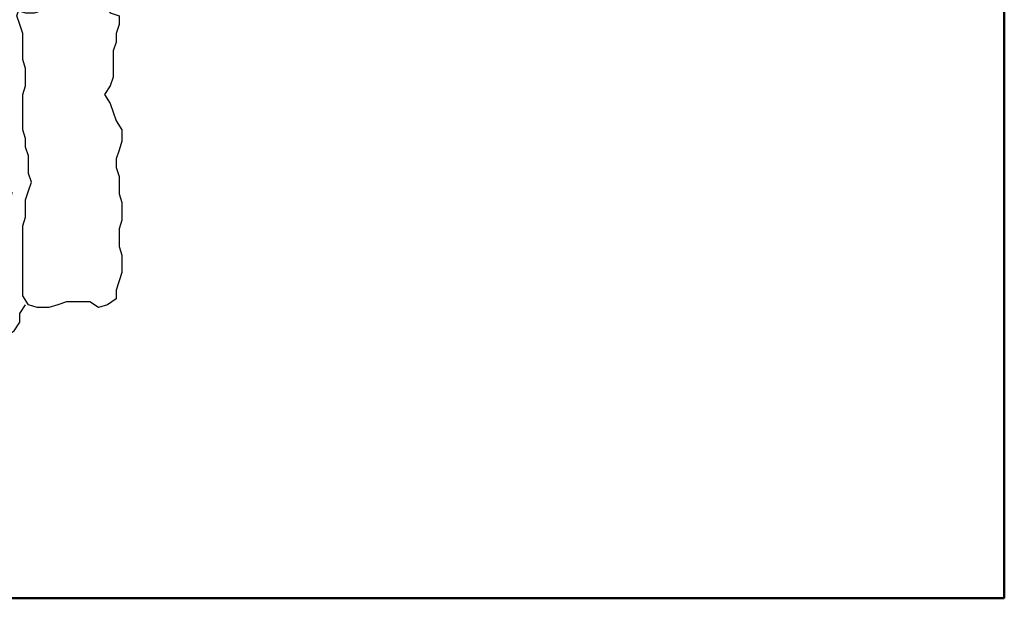
# Model space of a CAD drawing. Units: millimetres. Extents: x -857 to 54106, y -13666 to 13947.
# Tile 23 of 41: x 28540 to 29795, y 9579 to 10317. Entities that reach past the tile are written whole.
import ezdxf

# ---------------------------------------------------------------- set-up
doc = ezdxf.new("R2010")
doc.units = ezdxf.units.MM
doc.layers.add('A-FURN', color=21, linetype='Continuous', lineweight=18)
doc.layers.add('A-WALL', color=7, linetype='Continuous', lineweight=50)
doc.layers.add('TEFRIŞ', color=11, linetype='Continuous')

# ---------------------------------------------------------------- blocks, each defined once
blk = doc.blocks.new('26')
at = {"layer": 'TEFRIŞ'}
for p, q in [((-1589.6, -261.66), (-1588.12, -260.68)), ((-1588.12, -260.68), (-1586.16, -260.68)), ((-1586.16, -260.68), (-1584.68, -261.17)), ((-1577.3, -261.17), (-1575.83, -260.68)), ((-1575.83, -260.68), (-1572.87, -260.68)), ((-1572.87, -260.68), (-1571.4, -261.17)), ((-1568.45, -261.17), (-1566.97, -260.68)), ((-1566.97, -260.68), (-1564.02, -260.68)), ((-1564.02, -260.68), (-1561.07, -261.66)), ((-1607.8, -262.65), (-1607.31, -261.17)), ((-1607.31, -261.17), (-1605.84, -261.17)), ((-1605.84, -261.17), (-1604.36, -261.66)), ((-1604.36, -261.66), (-1602.88, -261.66)), ((-1602.88, -261.66), (-1601.41, -262.16)), ((-1601.41, -262.16), (-1596.98, -262.16)), ((-1596.98, -262.16), (-1595.5, -262.65)), ((-1592.55, -262.65), (-1591.08, -262.16)), ((-1591.08, -262.16), (-1589.6, -261.66)), ((-1584.68, -261.17), (-1583.21, -261.66)), ((-1583.21, -261.66), (-1581.73, -261.66)), ((-1581.73, -261.66), (-1580.25, -261.17)), ((-1580.25, -261.17), (-1577.3, -261.17)), ((-1571.4, -261.17), (-1568.45, -261.17)), ((-1561.07, -261.66), (-1559.59, -261.66)), ((-1559.59, -261.66), (-1558.61, -263.14)), ((-1609.77, -265.11), (-1609.28, -263.63)), ((-1609.28, -263.63), (-1607.8, -262.65)), ((-1595.5, -262.65), (-1594.03, -263.63)), ((-1594.03, -263.63), (-1592.55, -262.65)), ((-1558.61, -263.14), (-1558.12, -264.62)), ((-1609.77, -271.02), (-1609.77, -265.11)), ((-1558.12, -264.62), (-1559.1, -266.1)), ((-1559.1, -266.1), (-1559.1, -270.03)), ((-1559.1, -270.03), (-1558.61, -271.51)), ((-1609.28, -272.49), (-1609.77, -271.02)), ((-1558.61, -271.51), (-1558.12, -272.99)), ((-1608.29, -273.97), (-1609.28, -272.49)), ((-1607.8, -275.45), (-1608.29, -273.97)), ((-1558.12, -272.99), (-1558.12, -274.96)), ((-1607.8, -276.93), (-1607.8, -275.45)), ((-1558.12, -274.96), (-1558.61, -276.43)), ((-1608.29, -278.4), (-1607.8, -276.93)), ((-1598.46, -276.93), (-1599.93, -277.42)), ((-1595.5, -276.93), (-1598.46, -276.93)), ((-1594.03, -277.42), (-1595.5, -276.93)), ((-1586.65, -276.93), (-1588.12, -277.42)), ((-1585.17, -276.93), (-1586.65, -276.93)), ((-1583.7, -276.43), (-1585.17, -276.93)), ((-1580.75, -276.43), (-1583.7, -276.43)), ((-1579.27, -275.94), (-1580.75, -276.43)), ((-1577.79, -276.43), (-1579.27, -275.94)), ((-1576.32, -276.93), (-1577.79, -276.43)), ((-1573.37, -276.93), (-1576.32, -276.93)), ((-1571.89, -277.42), (-1573.37, -276.93)), ((-1558.61, -276.43), (-1560.08, -277.42)), ((-1557.13, -277.91), (-1558.61, -276.93)), ((-1613.21, -278.89), (-1613.71, -280.37)), ((-1611.74, -277.42), (-1613.21, -278.89)), ((-1610.26, -277.91), (-1611.74, -277.42)), ((-1608.79, -277.91), (-1610.26, -277.91)), ((-1607.31, -278.4), (-1608.79, -277.91)), ((-1605.84, -277.91), (-1607.31, -278.4)), ((-1604.36, -277.42), (-1605.84, -277.91)), ((-1599.93, -277.42), (-1604.36, -277.42)), ((-1588.12, -277.42), (-1594.03, -277.42)), ((-1560.08, -277.42), (-1571.89, -277.42)), ((-1555.66, -277.91), (-1557.13, -277.91)), ((-1554.18, -278.89), (-1555.66, -277.91)), ((-1553.2, -280.37), (-1554.18, -278.89)), ((-1613.71, -280.37), (-1614.69, -281.85)), ((-1577.69, -280.04), (-1577.46, -279.11)), ((-1577.69, -281.2), (-1577.69, -280.04)), ((-1577.23, -279.34), (-1576.07, -279.57)), ((-1576.07, -279.57), (-1573.75, -279.57)), ((-1573.75, -279.57), (-1572.59, -280.27)), ((-1572.59, -280.27), (-1571.43, -280.5)), ((-1571.43, -280.5), (-1570.27, -280.27)), ((-1570.27, -280.27), (-1569.12, -279.81)), ((-1569.12, -279.81), (-1567.96, -279.81)), ((-1567.96, -279.81), (-1566.8, -280.04)), ((-1566.8, -280.04), (-1565.64, -280.5)), ((-1565.64, -280.5), (-1563.32, -280.5)), ((-1563.32, -280.5), (-1562.16, -280.27)), ((-1562.16, -280.27), (-1561, -280.5)), ((-1561, -280.5), (-1559.84, -281.2)), ((-1553.2, -281.85), (-1553.2, -280.37)), ((-1614.69, -281.85), (-1614.69, -283.33)), ((-1578.16, -282.36), (-1577.69, -281.2)), ((-1572.36, -281.89), (-1573.29, -283.05)), ((-1572.13, -280.73), (-1572.36, -281.89)), ((-1571.66, -280.73), (-1570.51, -281.43)), ((-1570.51, -281.43), (-1569.35, -281.89)), ((-1569.35, -281.89), (-1568.19, -282.13)), ((-1568.19, -282.13), (-1567.03, -282.36)), ((-1559.84, -281.2), (-1558.68, -281.43)), ((-1558.68, -281.43), (-1558.22, -282.59)), ((-1553.69, -283.33), (-1553.2, -281.85)), ((-1552.21, -282.34), (-1550.74, -281.36)), ((-1550.74, -281.36), (-1549.26, -281.36)), ((-1549.26, -281.36), (-1547.78, -281.85)), ((-1547.78, -281.85), (-1546.31, -282.34)), ((-1614.69, -283.33), (-1615.18, -284.8)), ((-1578.62, -284.68), (-1578.39, -283.52)), ((-1578.39, -283.52), (-1578.16, -282.36)), ((-1573.29, -283.05), (-1573.29, -284.21)), ((-1567.03, -282.36), (-1565.87, -282.36)), ((-1565.87, -282.36), (-1564.71, -283.05)), ((-1564.71, -283.05), (-1563.55, -283.98)), ((-1558.22, -282.59), (-1558.45, -284.68)), ((-1554.18, -284.8), (-1553.69, -283.33)), ((-1553.69, -282.83), (-1552.21, -282.34)), ((-1546.31, -282.34), (-1544.83, -282.83)), ((-1544.83, -282.83), (-1543.36, -282.83)), ((-1543.36, -282.83), (-1541.88, -282.34)), ((-1541.88, -282.34), (-1540.9, -283.82)), ((-1540.9, -283.82), (-1540.4, -285.29)), ((-1615.18, -284.8), (-1615.18, -286.28)), ((-1578.62, -285.84), (-1578.62, -284.68)), ((-1573.29, -284.21), (-1572.13, -284.91)), ((-1572.13, -284.91), (-1570.97, -285.14)), ((-1570.97, -285.14), (-1569.81, -284.91)), ((-1569.81, -284.91), (-1568.65, -284.91)), ((-1568.65, -284.91), (-1567.49, -284.68)), ((-1567.49, -284.68), (-1566.33, -284.45)), ((-1566.33, -284.45), (-1565.17, -285.37)), ((-1565.17, -285.37), (-1564.25, -286.53)), ((-1563.55, -283.98), (-1562.39, -284.91)), ((-1562.39, -284.91), (-1561.7, -286.07)), ((-1558.45, -284.68), (-1558.68, -285.84)), ((-1555.16, -286.28), (-1554.18, -284.8)), ((-1540.4, -285.29), (-1540.4, -286.77)), ((-1615.18, -286.28), (-1614.69, -287.76)), ((-1578.39, -287), (-1578.62, -285.84)), ((-1577.69, -288.16), (-1578.39, -287)), ((-1564.25, -286.53), (-1563.09, -287.46)), ((-1561.7, -286.07), (-1561.47, -287.23)), ((-1561.47, -287.23), (-1561.23, -288.39)), ((-1558.68, -285.84), (-1558.68, -287)), ((-1558.68, -287), (-1558.45, -288.39)), ((-1555.66, -287.76), (-1555.16, -286.28)), ((-1540.4, -286.77), (-1540.9, -288.25)), ((-1614.69, -287.76), (-1614.69, -304.99)), ((-1576.76, -289.32), (-1577.69, -288.16)), ((-1563.09, -287.46), (-1562.86, -288.62)), ((-1562.86, -288.62), (-1562.86, -290.94)), ((-1561.23, -288.39), (-1561.23, -291.87)), ((-1558.45, -288.39), (-1558.45, -289.78)), ((-1555.66, -292.19), (-1555.66, -287.76)), ((-1540.9, -288.25), (-1540.9, -290.22)), ((-1576.3, -290.48), (-1576.76, -289.32)), ((-1576.07, -292.8), (-1576.3, -290.48)), ((-1558.45, -289.78), (-1558.22, -291.64)), ((-1540.9, -290.22), (-1540.4, -291.69)), ((-1563.32, -292.1), (-1563.78, -293.26)), ((-1562.86, -290.94), (-1563.32, -292.1)), ((-1561.23, -291.87), (-1560.77, -293.03)), ((-1558.22, -291.64), (-1557.76, -292.8)), ((-1555.16, -293.66), (-1555.66, -292.19)), ((-1540.4, -291.69), (-1540.4, -293.17)), ((-1576.07, -294.19), (-1576.07, -292.8)), ((-1563.78, -293.26), (-1563.55, -294.42)), ((-1560.77, -293.03), (-1560.31, -294.19)), ((-1557.76, -292.8), (-1557.76, -295.12)), ((-1554.67, -295.63), (-1555.16, -293.66)), ((-1540.4, -293.17), (-1539.91, -294.65)), ((-1576.76, -296.74), (-1576.3, -295.58)), ((-1576.3, -295.58), (-1576.07, -294.19)), ((-1563.55, -294.42), (-1562.39, -295.35)), ((-1562.39, -295.35), (-1561.23, -296.04)), ((-1560.31, -294.19), (-1560.07, -295.58)), ((-1560.07, -295.58), (-1559.84, -296.74)), ((-1557.76, -295.12), (-1558.92, -295.81)), ((-1539.91, -294.65), (-1539.42, -296.12)), ((-1577, -298.13), (-1576.76, -296.74)), ((-1561.23, -296.04), (-1560.07, -296.74)), ((-1559.84, -297.2), (-1560.77, -298.36)), ((-1560.07, -296.74), (-1559.61, -296.97)), ((-1558.92, -295.81), (-1559.84, -297.2)), ((-1554.67, -297.6), (-1554.67, -295.63)), ((-1539.42, -296.12), (-1538.93, -297.6)), ((-1576.53, -299.29), (-1577, -298.13)), ((-1574.21, -298.83), (-1575.37, -299.29)), ((-1573.06, -298.83), (-1574.21, -298.83)), ((-1571.9, -298.59), (-1573.06, -298.83)), ((-1570.74, -298.13), (-1571.9, -298.59)), ((-1569.58, -297.67), (-1570.74, -298.13)), ((-1568.19, -297.67), (-1569.58, -297.67)), ((-1567.03, -297.43), (-1568.19, -297.67)), ((-1565.87, -297.43), (-1567.03, -297.43)), ((-1564.48, -297.67), (-1565.87, -297.43)), ((-1563.09, -298.13), (-1564.48, -297.67)), ((-1561.93, -298.59), (-1563.09, -298.13)), ((-1560.77, -298.36), (-1561.93, -298.59)), ((-1554.18, -299.08), (-1554.67, -297.6)), ((-1538.93, -297.6), (-1538.93, -302.03)), ((-1575.37, -299.29), (-1576.53, -299.29)), ((-1554.18, -303.51), (-1554.18, -299.08)), ((-1538.93, -302.03), (-1539.42, -303.51)), ((-1553.69, -304.99), (-1554.18, -303.51)), ((-1539.42, -303.51), (-1539.91, -304.99)), ((-1614.69, -304.99), (-1614.2, -306.46)), ((-1553.69, -307.94), (-1553.69, -304.99)), ((-1539.91, -304.99), (-1539.91, -309.42)), ((-1614.2, -306.46), (-1614.2, -323.69)), ((-1554.18, -309.42), (-1553.69, -307.94)), ((-1554.18, -311.39), (-1554.18, -309.42)), ((-1539.91, -309.42), (-1539.42, -310.89)), ((-1554.67, -312.86), (-1554.18, -311.39)), ((-1539.42, -310.89), (-1538.93, -312.37)), ((-1555.16, -314.34), (-1554.67, -312.86)), ((-1538.93, -312.37), (-1538.44, -313.85)), ((-1538.44, -313.85), (-1537.95, -315.32)), ((-1555.16, -325.17), (-1555.16, -314.34)), ((-1537.95, -315.32), (-1537.95, -321.23)), ((-1537.95, -321.23), (-1538.44, -322.71)), ((-1614.2, -323.69), (-1613.71, -325.17)), ((-1538.44, -322.71), (-1538.44, -327.14)), ((-1613.71, -325.17), (-1613.71, -329.6)), ((-1554.67, -326.65), (-1555.16, -325.17)), ((-1554.18, -328.12), (-1554.67, -326.65)), ((-1538.44, -327.14), (-1538.93, -328.62)), ((-1553.69, -329.6), (-1554.18, -328.12)), ((-1538.93, -328.62), (-1538.93, -330.09)), ((-1613.71, -329.6), (-1614.2, -331.08)), ((-1553.13, -331.91), (-1553.13, -329.57)), ((-1538.93, -330.09), (-1539.91, -331.57)), ((-1614.2, -331.08), (-1614.69, -332.55)), ((-1552.79, -331.91), (-1553.13, -331.91)), ((-1552.79, -332.91), (-1552.79, -331.91)), ((-1540.13, -331.91), (-1540.13, -333.91)), ((-1614.69, -332.55), (-1614.69, -334.03)), ((-1552.46, -332.91), (-1552.79, -332.91)), ((-1552.46, -334.91), (-1552.46, -332.91)), ((-1614.69, -334.03), (-1613.21, -334.52)), ((-1613.21, -334.52), (-1611.74, -335.02)), ((-1611.74, -335.02), (-1610.75, -336.49)), ((-1552.79, -335.91), (-1552.79, -334.91)), ((-1552.79, -334.91), (-1552.46, -334.91)), ((-1540.46, -334.91), (-1541.13, -334.91)), ((-1541.13, -334.91), (-1541.13, -335.91)), ((-1540.13, -333.91), (-1540.46, -333.91)), ((-1540.46, -333.91), (-1540.46, -334.91)), ((-1610.75, -336.49), (-1609.77, -337.97)), ((-1607.45, -338.24), (-1607.45, -336.58)), ((-1607.45, -336.58), (-1605.78, -336.58)), ((-1605.78, -336.58), (-1605.78, -336.24)), ((-1605.78, -336.24), (-1604.78, -336.24)), ((-1604.78, -336.24), (-1604.78, -335.91)), ((-1604.78, -335.91), (-1602.79, -335.91)), ((-1602.79, -335.91), (-1602.79, -336.24)), ((-1602.79, -336.24), (-1601.45, -336.24)), ((-1601.45, -336.24), (-1601.45, -336.58)), ((-1601.45, -336.58), (-1599.45, -336.58)), ((-1599.45, -336.58), (-1599.45, -336.91)), ((-1599.45, -336.91), (-1598.45, -336.91)), ((-1598.45, -336.91), (-1598.45, -337.24)), ((-1553.46, -337.91), (-1553.46, -335.91)), ((-1553.46, -335.91), (-1552.79, -335.91)), ((-1550.8, -337.58), (-1550.8, -336.91)), ((-1550.8, -336.91), (-1549.8, -336.91)), ((-1549.8, -336.91), (-1549.8, -336.24)), ((-1549.8, -336.24), (-1547.8, -336.24)), ((-1547.8, -336.24), (-1547.8, -337.58)), ((-1541.46, -336.91), (-1541.8, -336.91)), ((-1541.8, -336.91), (-1541.8, -337.91)), ((-1541.13, -335.91), (-1541.46, -335.91)), ((-1541.46, -335.91), (-1541.46, -336.91)), ((-1612.74, -337.78), (-1614.21, -339.26)), ((-1611.26, -338.27), (-1612.74, -337.78)), ((-1609.79, -338.27), (-1611.26, -338.27)), ((-1609.45, -338.58), (-1608.45, -338.58)), ((-1608.45, -338.58), (-1608.45, -338.24)), ((-1608.45, -338.24), (-1607.45, -338.24)), ((-1598.45, -337.24), (-1597.12, -337.24)), ((-1597.12, -337.24), (-1597.12, -337.58)), ((-1597.12, -337.58), (-1596.12, -337.58)), ((-1596.12, -337.58), (-1596.12, -338.24)), ((-1596.12, -338.24), (-1595.12, -338.24)), ((-1595.12, -338.24), (-1595.12, -338.58)), ((-1595.12, -338.58), (-1593.12, -338.58)), ((-1593.12, -338.58), (-1593.12, -338.91)), ((-1568.13, -338.91), (-1568.13, -338.58)), ((-1568.13, -338.58), (-1566.13, -338.58)), ((-1566.13, -338.58), (-1566.13, -338.24)), ((-1566.13, -338.24), (-1564.13, -338.24)), ((-1564.13, -338.24), (-1564.13, -337.91)), ((-1564.13, -337.91), (-1561.79, -337.91)), ((-1561.79, -337.91), (-1561.79, -338.24)), ((-1561.79, -338.24), (-1557.13, -338.24)), ((-1557.13, -338.24), (-1557.13, -337.91)), ((-1557.13, -337.91), (-1553.79, -337.91)), ((-1553.79, -337.91), (-1553.79, -337.58)), ((-1552.79, -337.58), (-1553.13, -337.58)), ((-1553.13, -337.58), (-1553.13, -337.91)), ((-1552.79, -338.58), (-1552.79, -337.58)), ((-1552.79, -337.58), (-1550.8, -337.58)), ((-1552.46, -338.58), (-1552.79, -338.58)), ((-1552.46, -339.58), (-1552.46, -338.58)), ((-1547.8, -337.58), (-1546.13, -337.58)), ((-1546.13, -337.58), (-1546.13, -337.91)), ((-1546.13, -337.91), (-1545.13, -337.91)), ((-1545.13, -337.91), (-1545.13, -338.58)), ((-1545.13, -338.58), (-1543.13, -338.58)), ((-1543.13, -338.58), (-1543.13, -338.91)), ((-1541.8, -337.91), (-1542.13, -337.91)), ((-1542.13, -337.91), (-1542.13, -338.91)), ((-1614.21, -339.26), (-1614.71, -340.73)), ((-1593.12, -338.91), (-1589.12, -338.91)), ((-1589.12, -338.91), (-1589.12, -339.25)), ((-1589.12, -339.25), (-1587.12, -339.25)), ((-1587.12, -339.25), (-1587.12, -339.58)), ((-1587.12, -339.58), (-1577.46, -339.58)), ((-1577.46, -339.58), (-1577.46, -339.25)), ((-1577.46, -339.25), (-1574.46, -339.25)), ((-1574.46, -339.25), (-1574.46, -338.91)), ((-1574.46, -338.91), (-1568.13, -338.91)), ((-1552.13, -339.58), (-1552.46, -339.58)), ((-1552.13, -340.58), (-1552.13, -339.58)), ((-1543.13, -338.91), (-1542.8, -338.91)), ((-1542.8, -339.91), (-1543.13, -339.91)), ((-1543.13, -339.91), (-1543.13, -340.91)), ((-1542.13, -338.91), (-1542.8, -338.91)), ((-1542.8, -338.91), (-1542.8, -339.91)), ((-1614.71, -340.73), (-1615.69, -342.21)), ((-1551.8, -340.58), (-1552.13, -340.58)), ((-1551.8, -342.58), (-1551.8, -340.58)), ((-1543.13, -340.91), (-1542.8, -340.91)), ((-1542.8, -340.91), (-1542.8, -341.91)), ((-1542.8, -341.91), (-1542.13, -341.91)), ((-1542.13, -341.91), (-1542.13, -342.91)), ((-1615.69, -343.69), (-1616.18, -345.16)), ((-1615.69, -342.21), (-1615.69, -343.69)), ((-1552.46, -344.25), (-1552.46, -342.58)), ((-1552.46, -342.58), (-1551.8, -342.58)), ((-1542.13, -342.91), (-1541.8, -342.91)), ((-1541.88, -343.7), (-1540.9, -345.18)), ((-1616.18, -345.16), (-1616.18, -346.64)), ((-1554.18, -346.17), (-1553.69, -344.69)), ((-1553.46, -344.25), (-1552.46, -344.25)), ((-1540.9, -345.18), (-1540.4, -346.66)), ((-1616.18, -346.64), (-1615.69, -348.12)), ((-1555.16, -347.64), (-1554.18, -346.17)), ((-1540.4, -346.66), (-1540.4, -348.13)), ((-1615.69, -348.12), (-1615.69, -365.35)), ((-1555.66, -349.12), (-1555.16, -347.64)), ((-1540.4, -348.13), (-1540.9, -349.61)), ((-1555.66, -353.55), (-1555.66, -349.12)), ((-1540.9, -349.61), (-1540.9, -351.58)), ((-1540.9, -351.58), (-1540.4, -353.06)), ((-1555.16, -355.03), (-1555.66, -353.55)), ((-1540.4, -353.06), (-1540.4, -354.53)), ((-1554.67, -357), (-1555.16, -355.03)), ((-1540.4, -354.53), (-1539.91, -356.01)), ((-1554.67, -358.96), (-1554.67, -357)), ((-1539.91, -356.01), (-1539.42, -357.49)), ((-1539.42, -357.49), (-1538.93, -358.96)), ((-1554.18, -360.44), (-1554.67, -358.96)), ((-1538.93, -358.96), (-1538.93, -363.4)), ((-1554.18, -364.87), (-1554.18, -360.44)), ((-1538.93, -363.4), (-1539.42, -364.87)), ((-1553.69, -366.35), (-1554.18, -364.87)), ((-1539.42, -364.87), (-1539.91, -366.35)), ((-1615.69, -365.35), (-1615.2, -366.83)), ((-1615.2, -366.83), (-1615.2, -384.06)), ((-1553.69, -369.3), (-1553.69, -366.35)), ((-1539.91, -366.35), (-1539.91, -370.78)), ((-1554.18, -370.78), (-1553.69, -369.3)), ((-1554.18, -372.75), (-1554.18, -370.78)), ((-1539.91, -370.78), (-1539.42, -372.26)), ((-1554.67, -374.23), (-1554.18, -372.75)), ((-1539.42, -372.26), (-1538.93, -373.73)), ((-1576.53, -374.2), (-1577, -375.36)), ((-1575.37, -374.2), (-1576.53, -374.2)), ((-1574.21, -374.66), (-1575.37, -374.2)), ((-1573.06, -374.66), (-1574.21, -374.66)), ((-1571.9, -374.89), (-1573.06, -374.66)), ((-1570.74, -375.36), (-1571.9, -374.89)), ((-1561.93, -374.89), (-1563.09, -375.36)), ((-1560.77, -375.12), (-1561.93, -374.89)), ((-1559.84, -376.28), (-1560.77, -375.12)), ((-1555.16, -375.7), (-1554.67, -374.23)), ((-1538.93, -373.73), (-1538.44, -375.21)), ((-1538.44, -375.21), (-1537.95, -376.69)), ((-1577, -375.36), (-1576.76, -376.75)), ((-1576.76, -376.75), (-1576.3, -377.91)), ((-1569.58, -375.82), (-1570.74, -375.36)), ((-1568.19, -375.82), (-1569.58, -375.82)), ((-1567.03, -376.05), (-1568.19, -375.82)), ((-1565.87, -376.05), (-1567.03, -376.05)), ((-1564.48, -375.82), (-1565.87, -376.05)), ((-1563.09, -375.36), (-1564.48, -375.82)), ((-1561.23, -377.44), (-1560.07, -376.75)), ((-1560.07, -376.75), (-1559.61, -376.52)), ((-1560.07, -377.91), (-1559.84, -376.75)), ((-1558.92, -377.68), (-1559.84, -376.28)), ((-1555.16, -386.53), (-1555.16, -375.7)), ((-1537.95, -376.69), (-1537.95, -382.59)), ((-1576.3, -377.91), (-1576.07, -379.3)), ((-1563.55, -379.07), (-1562.39, -378.14)), ((-1562.39, -378.14), (-1561.23, -377.44)), ((-1560.31, -379.3), (-1560.07, -377.91)), ((-1557.76, -378.37), (-1558.92, -377.68)), ((-1557.76, -380.69), (-1557.76, -378.37)), ((-1576.07, -379.3), (-1576.07, -380.69)), ((-1563.78, -380.23), (-1563.55, -379.07)), ((-1563.32, -381.39), (-1563.78, -380.23)), ((-1560.77, -380.46), (-1560.31, -379.3)), ((-1576.07, -380.69), (-1576.3, -383.01)), ((-1562.86, -382.55), (-1563.32, -381.39)), ((-1561.23, -381.62), (-1560.77, -380.46)), ((-1561.23, -385.1), (-1561.23, -381.62)), ((-1558.45, -383.71), (-1558.22, -381.85)), ((-1558.22, -381.85), (-1557.76, -380.69)), ((-1576.3, -383.01), (-1576.76, -384.17)), ((-1562.86, -384.87), (-1562.86, -382.55)), ((-1537.95, -382.59), (-1538.44, -384.07)), ((-1615.2, -384.06), (-1614.71, -385.53)), ((-1576.76, -384.17), (-1577.69, -385.33)), ((-1563.09, -386.03), (-1562.86, -384.87)), ((-1561.47, -386.26), (-1561.23, -385.1)), ((-1558.68, -386.49), (-1558.45, -385.1)), ((-1558.45, -385.1), (-1558.45, -383.71)), ((-1538.44, -384.07), (-1538.44, -388.5)), ((-1614.71, -385.53), (-1614.71, -389.96)), ((-1578.39, -386.49), (-1578.62, -387.65)), ((-1577.69, -385.33), (-1578.39, -386.49)), ((-1564.25, -386.95), (-1563.09, -386.03)), ((-1561.7, -387.42), (-1561.47, -386.26)), ((-1558.68, -387.65), (-1558.68, -386.49)), ((-1554.67, -388.01), (-1555.16, -386.53)), ((-1578.62, -387.65), (-1578.62, -388.81)), ((-1573.29, -389.27), (-1572.13, -388.58)), ((-1572.13, -388.58), (-1570.97, -388.35)), ((-1570.97, -388.35), (-1569.81, -388.58)), ((-1569.81, -388.58), (-1568.65, -388.58)), ((-1568.65, -388.58), (-1567.49, -388.81)), ((-1566.33, -389.04), (-1565.17, -388.11)), ((-1565.17, -388.11), (-1564.25, -386.95)), ((-1563.55, -389.51), (-1562.39, -388.58)), ((-1562.39, -388.58), (-1561.7, -387.42)), ((-1558.45, -388.81), (-1558.68, -387.65)), ((-1554.18, -389.49), (-1554.67, -388.01)), ((-1538.44, -388.5), (-1538.93, -389.98)), ((-1614.71, -389.96), (-1615.2, -391.44)), ((-1578.62, -388.81), (-1578.39, -389.97)), ((-1578.39, -389.97), (-1578.16, -391.13)), ((-1573.29, -390.43), (-1573.29, -389.27)), ((-1567.49, -388.81), (-1566.33, -389.04)), ((-1564.71, -390.43), (-1563.55, -389.51)), ((-1558.22, -390.9), (-1558.45, -388.81)), ((-1553.69, -390.96), (-1554.18, -389.49)), ((-1538.93, -389.98), (-1538.93, -391.46)), ((-1615.2, -391.44), (-1615.69, -392.92)), ((-1578.16, -391.13), (-1577.69, -392.29)), ((-1572.36, -391.59), (-1573.29, -390.43)), ((-1572.13, -392.75), (-1572.36, -391.59)), ((-1570.51, -392.06), (-1569.35, -391.59)), ((-1569.35, -391.59), (-1568.19, -391.36)), ((-1568.19, -391.36), (-1567.03, -391.13)), ((-1567.03, -391.13), (-1565.87, -391.13)), ((-1565.87, -391.13), (-1564.71, -390.43)), ((-1558.68, -392.06), (-1558.22, -390.9)), ((-1538.93, -391.46), (-1539.91, -392.93)), ((-1615.69, -392.92), (-1615.69, -394.39)), ((-1577.69, -392.29), (-1577.69, -393.45)), ((-1577.69, -393.45), (-1577.46, -394.38)), ((-1573.75, -393.91), (-1572.59, -393.22)), ((-1572.59, -393.22), (-1571.43, -392.99)), ((-1571.66, -392.75), (-1570.51, -392.06)), ((-1571.43, -392.99), (-1570.27, -393.22)), ((-1570.27, -393.22), (-1569.12, -393.68)), ((-1567.96, -393.68), (-1566.8, -393.45)), ((-1566.8, -393.45), (-1565.64, -392.99)), ((-1565.64, -392.99), (-1563.32, -392.99)), ((-1563.32, -392.99), (-1562.16, -393.22)), ((-1562.16, -393.22), (-1561, -392.99)), ((-1561, -392.99), (-1559.84, -392.29)), ((-1559.84, -392.29), (-1558.68, -392.06)), ((-1553.13, -391.94), (-1553.13, -392.94)), ((-1553.13, -392.94), (-1552.46, -392.94)), ((-1553.13, -394.27), (-1553.13, -393.27)), ((-1553.13, -393.27), (-1552.46, -393.27)), ((-1552.46, -392.94), (-1552.46, -393.94)), ((-1540.46, -394.27), (-1540.46, -392.6)), ((-1540.46, -392.6), (-1539.8, -392.6)), ((-1615.69, -394.39), (-1614.21, -394.89)), ((-1614.21, -394.89), (-1612.74, -395.38)), ((-1577.23, -394.15), (-1576.07, -393.91)), ((-1576.07, -393.91), (-1573.75, -393.91)), ((-1569.12, -393.68), (-1567.96, -393.68)), ((-1556.13, -396.27), (-1556.13, -394.94)), ((-1556.13, -394.94), (-1554.13, -394.94)), ((-1554.13, -394.94), (-1554.13, -394.27)), ((-1554.13, -394.27), (-1553.13, -394.27)), ((-1552.46, -393.94), (-1550.46, -393.94)), ((-1550.46, -393.94), (-1550.46, -394.27)), ((-1550.46, -394.27), (-1546.46, -394.27)), ((-1546.46, -394.27), (-1546.46, -394.61)), ((-1546.46, -394.61), (-1544.46, -394.61)), ((-1544.46, -394.61), (-1544.46, -394.94)), ((-1544.46, -394.94), (-1543.46, -394.94)), ((-1543.46, -394.94), (-1543.46, -394.61)), ((-1543.46, -394.61), (-1541.46, -394.61)), ((-1541.46, -394.61), (-1541.46, -394.27)), ((-1541.46, -394.27), (-1540.46, -394.27)), ((-1612.74, -395.38), (-1611.75, -396.85)), ((-1611.75, -396.85), (-1610.77, -398.33)), ((-1563.53, -397.1), (-1562.05, -396.6)), ((-1562.05, -396.6), (-1560.58, -396.6)), ((-1560.58, -396.6), (-1559.1, -397.59)), ((-1557.13, -397.27), (-1557.13, -396.27)), ((-1557.13, -396.27), (-1556.13, -396.27)), ((-1609.77, -398.57), (-1608.29, -398.08)), ((-1608.29, -398.08), (-1606.82, -398.08)), ((-1606.82, -398.08), (-1605.34, -397.59)), ((-1605.34, -397.59), (-1585.66, -397.59)), ((-1585.66, -397.59), (-1584.19, -397.1)), ((-1584.19, -397.1), (-1579.76, -397.1)), ((-1579.76, -397.1), (-1578.29, -397.59)), ((-1578.29, -397.59), (-1573.86, -397.59)), ((-1573.86, -397.59), (-1572.38, -398.08)), ((-1572.38, -398.08), (-1569.43, -398.08)), ((-1569.43, -398.08), (-1567.95, -397.59)), ((-1567.95, -397.59), (-1565, -397.59)), ((-1565, -397.59), (-1563.53, -397.1)), ((-1558.61, -398.57), (-1559.1, -397.1)), ((-1559.1, -397.59), (-1557.62, -398.08)), ((-1558.46, -397.27), (-1557.13, -397.27)), ((-1608.79, -398.57), (-1609.77, -400.54)), ((-1559.1, -401.53), (-1558.61, -400.05)), ((-1558.61, -400.05), (-1558.61, -398.57)), ((-1609.77, -400.54), (-1611.25, -402.02)), ((-1560.08, -403), (-1559.1, -401.53)), ((-1611.25, -402.02), (-1612.23, -403.99)), ((-1560.08, -404.48), (-1560.08, -403)), ((-1612.23, -403.99), (-1612.23, -405.47)), ((-1559.59, -405.96), (-1560.08, -404.48)), ((-1612.23, -405.47), (-1611.25, -406.94)), ((-1558.61, -407.43), (-1559.59, -405.96)), ((-1611.25, -406.94), (-1609.77, -408.42)), ((-1609.77, -408.42), (-1609.28, -409.9)), ((-1558.61, -410.39), (-1558.61, -407.43)), ((-1609.28, -409.9), (-1608.29, -411.37)), ((-1608.29, -411.37), (-1606.82, -412.36)), ((-1593.54, -411.86), (-1592.06, -410.88)), ((-1592.06, -410.88), (-1590.58, -410.88)), ((-1590.58, -410.88), (-1589.11, -411.37)), ((-1589.11, -411.37), (-1587.63, -411.37)), ((-1587.63, -411.37), (-1586.16, -411.86)), ((-1569.43, -412.36), (-1566.48, -411.37)), ((-1566.48, -411.37), (-1565, -412.36)), ((-1559.1, -411.86), (-1558.61, -410.39)), ((-1606.82, -412.36), (-1603.87, -412.36)), ((-1603.87, -412.36), (-1602.39, -411.86)), ((-1602.39, -411.86), (-1593.54, -411.86)), ((-1586.16, -411.86), (-1584.68, -412.36)), ((-1584.68, -412.36), (-1583.21, -412.36)), ((-1583.21, -412.36), (-1581.73, -411.86)), ((-1581.73, -411.86), (-1579.76, -412.36)), ((-1579.76, -412.36), (-1578.29, -411.86)), ((-1578.29, -411.86), (-1576.81, -411.86)), ((-1576.81, -411.86), (-1575.33, -412.36)), ((-1575.33, -412.36), (-1573.86, -412.85)), ((-1573.86, -412.85), (-1572.38, -412.85)), ((-1572.38, -412.85), (-1570.91, -412.36)), ((-1570.91, -412.36), (-1569.43, -412.36)), ((-1565, -412.36), (-1560.58, -412.36)), ((-1560.58, -412.36), (-1559.1, -411.86))]:
    blk.add_line(p, q, dxfattribs=at)

msp = doc.modelspace()

# ---------------------------------------------------------------- linework, layer by layer
at = {"layer": 'A-WALL'}
for p, q in [((29795.079, 11628.89), (29795.079, 9579.231)), ((29795.079, 9579.231), (27188.012, 9579.231)), ((28170.079, 9579.231), (28870.079, 9579.231))]:
    msp.add_line(p, q, dxfattribs=at)

# ---------------------------------------------------------------- block references
at = {"layer": 'A-FURN', "xscale": 7.559220362162901, "yscale": 7.559220362162901, "zscale": 7.559220362162901, "rotation": 270}
msp.add_blockref('26', (30640.69, -1828.483), dxfattribs=at)

doc.saveas('drawing.dxf')
